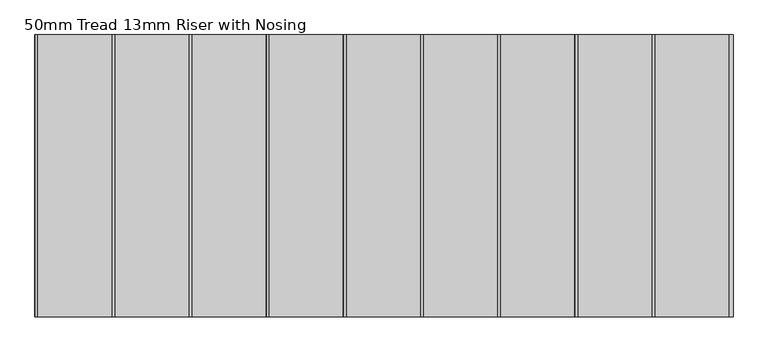
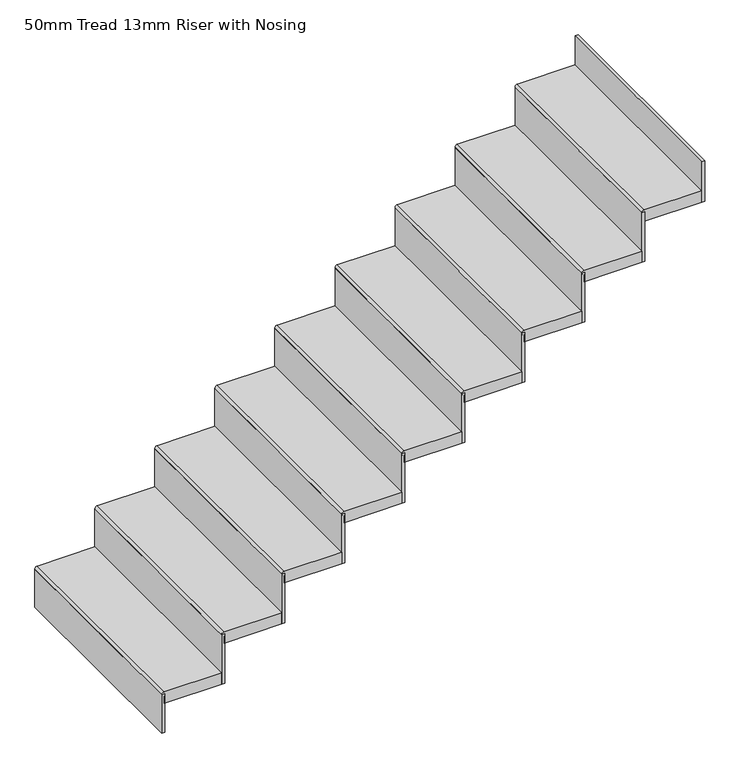
"""IFC4 building model written with IfcOpenShell, lengths in millimetres: stair flight geometry, 50mm Tread 13mm Riser with Nosing."""

from ifc_helpers import new_model, si_unit, point, frame, frame_2d, origin, origin_with_axes, place, context, project, spatial, polyline, circle_curve, trimmed, segment, composite_curve, outline, extrude, source, transform, mapped, element, save


def stair_flight_50mm_tread_13mm_riser_with_nosing_6f61a695(model_context):
    return source(origin(), model_context, "Body", "SweptSolid", [
        extrude(outline(polyline([(-9791.7282945, -3247.1921603), (-9804.2282945, -3247.1921603), (-9804.2282945, -2332.7921603), (-9791.7282945, -2332.7921603), (-9791.7282945, -3247.1921603)])), origin_with_axes(), (0.0, 0.0, 1.0), 167.8),
        extrude(outline(composite_curve([segment(polyline([(177.8, -9554.2282945), (177.8, -9794.2282945)]), True, "CONTINUOUS"), segment(trimmed(circle_curve(frame_2d((167.8, -9794.2282945)), 10.0), [point((177.8, -9794.2282945))], [point((157.8, -9794.2282945))], False, "CARTESIAN"), True, "CONTINUOUS"), segment(polyline([(157.8, -9794.2282945), (127.8, -9794.2282945), (127.8, -9554.2282945), (177.8, -9554.2282945)]), True, "CONTINUOUS")], self_intersect=False)), frame((0.0, -3247.1921603, 0.0), z_axis=(0.0, 1.0, 0.0), x_axis=(0.0, 0.0, 1.0)), (0.0, 0.0, 1.0), 914.4),
        extrude(outline(polyline([(-9541.7282945, -3247.1921603), (-9554.2282945, -3247.1921603), (-9554.2282945, -2332.7921603), (-9541.7282945, -2332.7921603), (-9541.7282945, -3247.1921603)])), frame((0.0, 0.0, 127.8), z_axis=(0.0, 0.0, 1.0), x_axis=(1.0, 0.0, 0.0)), (0.0, 0.0, 1.0), 217.8),
        extrude(outline(composite_curve([segment(polyline([(355.6, -9304.2282945), (355.6, -9544.2282945)]), True, "CONTINUOUS"), segment(trimmed(circle_curve(frame_2d((345.6, -9544.2282945)), 10.0), [point((355.6, -9544.2282945))], [point((335.6, -9544.2282945))], False, "CARTESIAN"), True, "CONTINUOUS"), segment(polyline([(335.6, -9544.2282945), (305.6, -9544.2282945), (305.6, -9304.2282945), (355.6, -9304.2282945)]), True, "CONTINUOUS")], self_intersect=False)), frame((0.0, -3247.1921603, 0.0), z_axis=(0.0, 1.0, 0.0), x_axis=(0.0, 0.0, 1.0)), (0.0, 0.0, 1.0), 914.4),
        extrude(outline(polyline([(-9291.7282945, -3247.1921603), (-9304.2282945, -3247.1921603), (-9304.2282945, -2332.7921603), (-9291.7282945, -2332.7921603), (-9291.7282945, -3247.1921603)])), frame((0.0, 0.0, 305.6), z_axis=(0.0, 0.0, 1.0), x_axis=(1.0, 0.0, 0.0)), (0.0, 0.0, 1.0), 217.8),
        extrude(outline(composite_curve([segment(polyline([(533.4, -9054.2282945), (533.4, -9294.2282945)]), True, "CONTINUOUS"), segment(trimmed(circle_curve(frame_2d((523.4, -9294.2282945)), 10.0), [point((533.4, -9294.2282945))], [point((513.4, -9294.2282945))], False, "CARTESIAN"), True, "CONTINUOUS"), segment(polyline([(513.4, -9294.2282945), (483.4, -9294.2282945), (483.4, -9054.2282945), (533.4, -9054.2282945)]), True, "CONTINUOUS")], self_intersect=False)), frame((0.0, -3247.1921603, 0.0), z_axis=(0.0, 1.0, 0.0), x_axis=(0.0, 0.0, 1.0)), (0.0, 0.0, 1.0), 914.4),
        extrude(outline(polyline([(-9041.7282945, -3247.1921603), (-9054.2282945, -3247.1921603), (-9054.2282945, -2332.7921603), (-9041.7282945, -2332.7921603), (-9041.7282945, -3247.1921603)])), frame((0.0, 0.0, 483.4), z_axis=(0.0, 0.0, 1.0), x_axis=(1.0, 0.0, 0.0)), (0.0, 0.0, 1.0), 217.8),
        extrude(outline(composite_curve([segment(polyline([(711.2, -8804.2282945), (711.2, -9044.2282945)]), True, "CONTINUOUS"), segment(trimmed(circle_curve(frame_2d((701.2, -9044.2282945)), 10.0), [point((711.2, -9044.2282945))], [point((691.2, -9044.2282945))], False, "CARTESIAN"), True, "CONTINUOUS"), segment(polyline([(691.2, -9044.2282945), (661.2, -9044.2282945), (661.2, -8804.2282945), (711.2, -8804.2282945)]), True, "CONTINUOUS")], self_intersect=False)), frame((0.0, -3247.1921603, 0.0), z_axis=(0.0, 1.0, 0.0), x_axis=(0.0, 0.0, 1.0)), (0.0, 0.0, 1.0), 914.4),
        extrude(outline(polyline([(-8791.7282945, -3247.1921603), (-8804.2282945, -3247.1921603), (-8804.2282945, -2332.7921603), (-8791.7282945, -2332.7921603), (-8791.7282945, -3247.1921603)])), frame((0.0, 0.0, 661.2), z_axis=(0.0, 0.0, 1.0), x_axis=(1.0, 0.0, 0.0)), (0.0, 0.0, 1.0), 217.8),
        extrude(outline(composite_curve([segment(polyline([(889.0, -8554.2282945), (889.0, -8794.2282945)]), True, "CONTINUOUS"), segment(trimmed(circle_curve(frame_2d((879.0, -8794.2282945)), 10.0), [point((889.0, -8794.2282945))], [point((869.0, -8794.2282945))], False, "CARTESIAN"), True, "CONTINUOUS"), segment(polyline([(869.0, -8794.2282945), (839.0, -8794.2282945), (839.0, -8554.2282945), (889.0, -8554.2282945)]), True, "CONTINUOUS")], self_intersect=False)), frame((0.0, -3247.1921603, 0.0), z_axis=(0.0, 1.0, 0.0), x_axis=(0.0, 0.0, 1.0)), (0.0, 0.0, 1.0), 914.4),
        extrude(outline(polyline([(-8541.7282945, -3247.1921603), (-8554.2282945, -3247.1921603), (-8554.2282945, -2332.7921603), (-8541.7282945, -2332.7921603), (-8541.7282945, -3247.1921603)])), frame((0.0, 0.0, 839.0), z_axis=(0.0, 0.0, 1.0), x_axis=(1.0, 0.0, 0.0)), (0.0, 0.0, 1.0), 217.8),
        extrude(outline(composite_curve([segment(polyline([(1066.8, -8304.2282945), (1066.8, -8544.2282945)]), True, "CONTINUOUS"), segment(trimmed(circle_curve(frame_2d((1056.8, -8544.2282945)), 10.0), [point((1066.8, -8544.2282945))], [point((1046.8, -8544.2282945))], False, "CARTESIAN"), True, "CONTINUOUS"), segment(polyline([(1046.8, -8544.2282945), (1016.8, -8544.2282945), (1016.8, -8304.2282945), (1066.8, -8304.2282945)]), True, "CONTINUOUS")], self_intersect=False)), frame((0.0, -3247.1921603, 0.0), z_axis=(0.0, 1.0, 0.0), x_axis=(0.0, 0.0, 1.0)), (0.0, 0.0, 1.0), 914.4),
        extrude(outline(polyline([(-8291.7282945, -3247.1921603), (-8304.2282945, -3247.1921603), (-8304.2282945, -2332.7921603), (-8291.7282945, -2332.7921603), (-8291.7282945, -3247.1921603)])), frame((0.0, 0.0, 1016.8), z_axis=(0.0, 0.0, 1.0), x_axis=(1.0, 0.0, 0.0)), (0.0, 0.0, 1.0), 217.8),
        extrude(outline(composite_curve([segment(polyline([(1244.6, -8054.2282945), (1244.6, -8294.2282945)]), True, "CONTINUOUS"), segment(trimmed(circle_curve(frame_2d((1234.6, -8294.2282945)), 10.0), [point((1244.6, -8294.2282945))], [point((1224.6, -8294.2282945))], False, "CARTESIAN"), True, "CONTINUOUS"), segment(polyline([(1224.6, -8294.2282945), (1194.6, -8294.2282945), (1194.6, -8054.2282945), (1244.6, -8054.2282945)]), True, "CONTINUOUS")], self_intersect=False)), frame((0.0, -3247.1921603, 0.0), z_axis=(0.0, 1.0, 0.0), x_axis=(0.0, 0.0, 1.0)), (0.0, 0.0, 1.0), 914.4),
        extrude(outline(polyline([(-8041.7282945, -3247.1921603), (-8054.2282945, -3247.1921603), (-8054.2282945, -2332.7921603), (-8041.7282945, -2332.7921603), (-8041.7282945, -3247.1921603)])), frame((0.0, 0.0, 1194.6), z_axis=(0.0, 0.0, 1.0), x_axis=(1.0, 0.0, 0.0)), (0.0, 0.0, 1.0), 217.8),
        extrude(outline(composite_curve([segment(polyline([(1422.4, -7804.2282945), (1422.4, -8044.2282945)]), True, "CONTINUOUS"), segment(trimmed(circle_curve(frame_2d((1412.4, -8044.2282945)), 10.0), [point((1422.4, -8044.2282945))], [point((1402.4, -8044.2282945))], False, "CARTESIAN"), True, "CONTINUOUS"), segment(polyline([(1402.4, -8044.2282945), (1372.4, -8044.2282945), (1372.4, -7804.2282945), (1422.4, -7804.2282945)]), True, "CONTINUOUS")], self_intersect=False)), frame((0.0, -3247.1921603, 0.0), z_axis=(0.0, 1.0, 0.0), x_axis=(0.0, 0.0, 1.0)), (0.0, 0.0, 1.0), 914.4),
        extrude(outline(polyline([(-7791.7282945, -3247.1921603), (-7804.2282945, -3247.1921603), (-7804.2282945, -2332.7921603), (-7791.7282945, -2332.7921603), (-7791.7282945, -3247.1921603)])), frame((0.0, 0.0, 1372.4), z_axis=(0.0, 0.0, 1.0), x_axis=(1.0, 0.0, 0.0)), (0.0, 0.0, 1.0), 217.8),
        extrude(outline(polyline([(-7541.7282945, -3247.1921603), (-7554.2282945, -3247.1921603), (-7554.2282945, -2332.7921603), (-7541.7282945, -2332.7921603), (-7541.7282945, -3247.1921603)])), frame((0.0, 0.0, 1550.2), z_axis=(0.0, 0.0, 1.0), x_axis=(1.0, 0.0, 0.0)), (0.0, 0.0, 1.0), 177.8),
        extrude(outline(composite_curve([segment(polyline([(1600.2, -7554.2282945), (1600.2, -7794.2282945)]), True, "CONTINUOUS"), segment(trimmed(circle_curve(frame_2d((1590.2, -7794.2282945)), 10.0), [point((1600.2, -7794.2282945))], [point((1580.2, -7794.2282945))], False, "CARTESIAN"), True, "CONTINUOUS"), segment(polyline([(1580.2, -7794.2282945), (1550.2, -7794.2282945), (1550.2, -7554.2282945), (1600.2, -7554.2282945)]), True, "CONTINUOUS")], self_intersect=False)), frame((0.0, -3247.1921603, 0.0), z_axis=(0.0, 1.0, 0.0), x_axis=(0.0, 0.0, 1.0)), (0.0, 0.0, 1.0), 914.4),
    ])


if __name__ == "__main__":
    model = new_model("IFC4")
    model_context = context("Model", 3, world=origin())
    ifc_project = project(units=[si_unit("LENGTHUNIT", "METRE", prefix="MILLI")], contexts=[model_context])
    site = spatial("IfcSite", under=ifc_project)
    building = spatial("IfcBuilding", under=site)
    placement = place(None, origin())
    stair_flight_50mm_tread_13mm_riser_with_nosing_shape = stair_flight_50mm_tread_13mm_riser_with_nosing_6f61a695(model_context)
    element("IfcStairFlight", 1, ObjectType="50mm Tread 13mm Riser with Nosing", at=placement, inside=building, context=model_context, shape_type="MappedRepresentation", body=[
        mapped(stair_flight_50mm_tread_13mm_riser_with_nosing_shape, transform((0.0, 0.0, 0.0), x_axis=(1.0, 0.0, 0.0), y_axis=(0.0, 1.0, 0.0), z_axis=(0.0, 0.0, 1.0))),
    ])
    save(model, "model.ifc")
